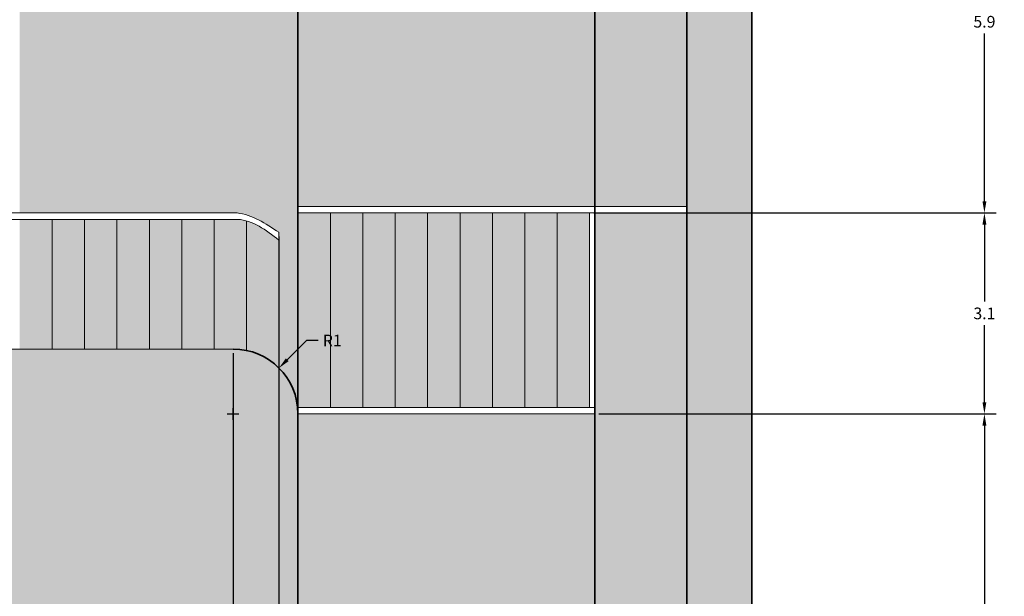
# Model space of a CAD drawing. Units: inches. Extents: x 18 to 59.8, y 2.7 to 81.2.
# Tile 9 of 9: x 44.6 to 59.8, y 45.6 to 54.5. Entities that reach past the tile are written whole.
import ezdxf

# ---------------------------------------------------------------- set-up
doc = ezdxf.new("R2010")
doc.units = ezdxf.units.IN
doc.header["$MEASUREMENT"] = 0
for name, color, linetype, lineweight in [('A-ANNO-DIMS', 2, 'Continuous', 18), ('A-ELEV', 7, 'Continuous', 35), ('A-ELEV-PATT', 8, 'Continuous', 13), ('A-ELEV-RAIL', 7, 'Continuous', 18)]:
    doc.layers.add(name, color=color, linetype=linetype, lineweight=lineweight)
doc.styles.get("Standard").update_dxf_attribs({"font": 'arial.ttf'})
doc.dimstyles.get("Standard").update_dxf_attribs({"dimtxt": 0.18, "dimasz": 0.18, "dimexe": 0.18, "dimexo": 0.0625, "dimgap": 0.09, "dimtad": 0, "dimtih": 1, "dimtoh": 1, "dimdec": 1, "dimzin": 0, "dimdsep": 46, "dimlunit": 3, "dimtxsty": 'Standard', "dimcen": 0.09, "dimadec": 0, "dimazin": 0, "dimtfac": 1, "dimtdec": 1, "dimtofl": 0, "dimtmove": 0, "dimatfit": 3, "dimfxl": 1, "dimtolj": 1, "dimtzin": 0, "dimarcsym": 0})

# ---------------------------------------------------------------- blocks, each defined once
blk = doc.blocks.new('*D17')
at = {"layer": 'A-ANNO-DIMS', "color": 0, "lineweight": -2, "transparency": 16777216}
for p, q in [((53.50256100000002, 48.44074800000003), (59.62997100000005, 48.44074800000003)), ((59.44997100000005, 48.26074800000003), (59.44997100000005, 43.74455863778991)), ((59.44997100000005, 38.86456300000001), (59.44997100000005, 43.38075236221011)), ((53.50256100000002, 38.68456300000001), (59.62997100000006, 38.68456300000001))]:
    blk.add_line(p, q, dxfattribs=at)
at = {"layer": 'A-ANNO-DIMS', "color": 0, "transparency": 16777216}
for points in [[(59.41997100000005, 48.26074800000003), (59.47997100000005, 48.26074800000003), (59.44997100000005, 48.44074800000003)], [(59.41997100000005, 38.86456300000001), (59.47997100000005, 38.86456300000001), (59.44997100000005, 38.68456300000001)]]:
    blk.add_solid(points, dxfattribs=at)
at = {"layer": 'Defpoints', "color": 0, "transparency": 16777216}
for p in [(53.44006100000003, 48.44074800000003), (59.44997100000005, 48.44074800000003), (53.44006100000003, 38.68456300000001)]:
    blk.add_point(p, dxfattribs=at)
at = {"layer": 'A-ANNO-DIMS', "color": 0, "transparency": 16777216, "insert": (59.44997100000005, 43.56265549999998), "char_height": 0.18, "attachment_point": 5}
blk.add_mtext('\\A1;9.756', dxfattribs=at)
blk = doc.blocks.new('*D18')
at = {"layer": 'A-ANNO-DIMS', "color": 0, "lineweight": -2, "transparency": 16777216}
for p, q in [((53.42247100000003, 51.54074800000003), (59.62997100000006, 51.54074800000003)), ((59.44997100000005, 51.36074800000002), (59.44997100000005, 50.17271252933154)), ((59.44997100000005, 48.62074800000002), (59.44997100000005, 49.80878347066851)), ((53.50256100000002, 48.44074800000003), (59.62997100000006, 48.44074800000003))]:
    blk.add_line(p, q, dxfattribs=at)
at = {"layer": 'A-ANNO-DIMS', "color": 0, "transparency": 16777216}
for points in [[(59.41997100000005, 51.36074800000002), (59.47997100000005, 51.36074800000002), (59.44997100000005, 51.54074800000003)], [(59.41997100000005, 48.62074800000002), (59.47997100000005, 48.62074800000002), (59.44997100000005, 48.44074800000003)]]:
    blk.add_solid(points, dxfattribs=at)
at = {"layer": 'Defpoints', "color": 0, "transparency": 16777216}
for p in [(53.35997100000003, 51.54074800000003), (59.44997100000005, 51.54074800000003), (53.44006100000003, 48.44074800000003)]:
    blk.add_point(p, dxfattribs=at)
at = {"layer": 'A-ANNO-DIMS', "color": 0, "transparency": 16777216, "insert": (59.44997100000005, 49.99074799999998), "char_height": 0.18, "attachment_point": 5}
blk.add_mtext('\\A1;3.1', dxfattribs=at)
blk = doc.blocks.new('*D19')
at = {"layer": 'A-ANNO-DIMS', "color": 0, "lineweight": -2, "transparency": 16777216}
for p, q in [((53.50256100000002, 57.44074800000003), (59.62997100000006, 57.44074800000003)), ((59.44997100000005, 57.26074800000002), (59.44997100000005, 54.67265113778992)), ((59.44997100000005, 51.72074800000003), (59.44997100000005, 54.30884486221012)), ((53.42247100000003, 51.54074800000003), (59.62997100000006, 51.54074800000003))]:
    blk.add_line(p, q, dxfattribs=at)
at = {"layer": 'A-ANNO-DIMS', "color": 0, "transparency": 16777216}
for points in [[(59.41997100000005, 57.26074800000002), (59.47997100000005, 57.26074800000002), (59.44997100000005, 57.44074800000003)], [(59.41997100000005, 51.72074800000003), (59.47997100000005, 51.72074800000003), (59.44997100000005, 51.54074800000003)]]:
    blk.add_solid(points, dxfattribs=at)
at = {"layer": 'Defpoints', "color": 0, "transparency": 16777216}
for p in [(53.44006100000003, 57.44074800000003), (59.44997100000005, 57.44074800000003), (53.35997100000003, 51.54074800000003)]:
    blk.add_point(p, dxfattribs=at)
at = {"layer": 'A-ANNO-DIMS', "color": 0, "transparency": 16777216, "insert": (59.44997100000005, 54.49074799999999), "char_height": 0.18, "attachment_point": 5}
blk.add_mtext('\\A1;5.9', dxfattribs=at)
blk = doc.blocks.new('*D51')
at = {"layer": 'A-ANNO-DIMS', "color": 0, "lineweight": -2, "transparency": 16777216}
for p, q in [((34.011642, 44.50324799999999), (34.011642, 81.210748)), ((48.859971, 43.503248), (48.859971, 81.210748)), ((34.191642, 81.03074799999999), (40.98046543587994, 81.03074799999999)), ((48.679971, 81.03074799999999), (41.89114756412005, 81.03074799999999))]:
    blk.add_line(p, q, dxfattribs=at)
at = {"layer": 'A-ANNO-DIMS', "color": 0, "transparency": 16777216}
for points in [[(34.191642, 81.060748), (34.191642, 81.00074799999999), (34.011642, 81.03074799999999)], [(48.679971, 81.060748), (48.679971, 81.00074799999999), (48.859971, 81.03074799999999)]]:
    blk.add_solid(points, dxfattribs=at)
at = {"layer": 'Defpoints', "color": 0, "transparency": 16777216}
for p in [(48.859971, 81.03074799999999), (34.011642, 44.440748), (48.859971, 43.440748)]:
    blk.add_point(p, dxfattribs=at)
at = {"layer": 'A-ANNO-DIMS', "color": 0, "transparency": 16777216, "insert": (41.43580649999999, 81.03074799999999), "char_height": 0.18, "attachment_point": 5}
blk.add_mtext('\\A1;14.848', dxfattribs=at)
blk = doc.blocks.new('*D61')
at = {"layer": 'A-ANNO-DIMS', "color": 0, "lineweight": -2, "transparency": 16777216}
for p, q in [((32.233824, 49.378248), (32.233824, 2.670748000000003)), ((47.859971, 49.378248), (47.859971, 2.670748000000003)), ((32.413824, 2.850747999999999), (39.59180200204638, 2.850747999999999)), ((47.679971, 2.850747999999999), (40.50199299795361, 2.850747999999999))]:
    blk.add_line(p, q, dxfattribs=at)
at = {"layer": 'A-ANNO-DIMS', "color": 0, "transparency": 16777216}
for points in [[(32.413824, 2.880747999999999), (32.413824, 2.820748), (32.233824, 2.850747999999999)], [(47.679971, 2.880747999999999), (47.679971, 2.820748), (47.859971, 2.850747999999999)]]:
    blk.add_solid(points, dxfattribs=at)
at = {"layer": 'Defpoints', "color": 0, "transparency": 16777216}
for p in [(32.233824, 49.440748), (47.859971, 49.440748), (47.859971, 2.850747999999999)]:
    blk.add_point(p, dxfattribs=at)
at = {"layer": 'A-ANNO-DIMS', "color": 0, "transparency": 16777216, "insert": (40.04689749999999, 2.850747999999999), "char_height": 0.18, "attachment_point": 5}
blk.add_mtext('\\A1;15.626', dxfattribs=at)
blk = doc.blocks.new('*D66')
at = {"layer": 'A-ANNO-DIMS', "color": 0, "lineweight": -2, "transparency": 16777216}
for p, q in [((28.803543, 51.378248), (28.803543, 2.670748000000003)), ((48.567078, 51.179103), (48.567078, 2.670748000000003)), ((28.983543, 2.850747999999999), (38.23052195975444, 2.850747999999999)), ((48.387078, 2.850747999999999), (39.14009904024556, 2.850747999999999))]:
    blk.add_line(p, q, dxfattribs=at)
at = {"layer": 'A-ANNO-DIMS', "color": 0, "transparency": 16777216}
for points in [[(28.983543, 2.880747999999999), (28.983543, 2.820748), (28.803543, 2.850747999999999)], [(48.387078, 2.880747999999999), (48.387078, 2.820748), (48.567078, 2.850747999999999)]]:
    blk.add_solid(points, dxfattribs=at)
at = {"layer": 'Defpoints', "color": 0, "transparency": 16777216}
for p in [(28.803543, 51.440748), (48.567078, 51.24160299999999), (48.567078, 2.850747999999999)]:
    blk.add_point(p, dxfattribs=at)
at = {"layer": 'A-ANNO-DIMS', "color": 0, "transparency": 16777216, "insert": (38.6853105, 2.850747999999999), "char_height": 0.18, "attachment_point": 5}
blk.add_mtext('\\A1;19.764', dxfattribs=at)
blk = doc.blocks.new('*D74')
at = {"layer": 'A-ANNO-DIMS', "color": 0, "lineweight": -2, "transparency": 16777216}
for p, q in [((48.99116316341159, 49.57229696346313), (48.69422514902348, 49.27526528903895)), ((49.1711631634116, 49.57229696346313), (48.99116316341159, 49.57229696346313)), ((47.859971, 48.35074800000001), (47.859971, 48.53074800000001)), ((47.769971, 48.44074800000001), (47.949971, 48.44074800000001))]:
    blk.add_line(p, q, dxfattribs=at)
at = {"layer": 'A-ANNO-DIMS', "color": 0, "transparency": 16777216}
blk.add_solid([(48.67300860085032, 49.29647514720953), (48.71544169719663, 49.25405543086837), (48.566966, 49.14796599999999)], dxfattribs=at)
at = {"layer": 'Defpoints', "color": 0, "transparency": 16777216}
for p in [(48.566966, 49.14796599999999), (47.85997100000001, 48.44074800000001)]:
    blk.add_point(p, dxfattribs=at)
at = {"layer": 'A-ANNO-DIMS', "color": 0, "transparency": 16777216, "insert": (49.38891896150163, 49.57229696346313), "char_height": 0.18, "attachment_point": 5}
blk.add_mtext('\\A1;R1', dxfattribs=at)

msp = doc.modelspace()

# ---------------------------------------------------------------- hatches: boundary and pattern name
at = {"layer": 'A-ELEV-PATT'}
h = msp.add_hatch(color=256, dxfattribs=at)
h.set_gradient(color1=(255, 255, 255), color2=(199, 200, 202))
h.paths.add_polyline_path([(38.85997087182833, 75.45212783007513, 0.4125526599533602), (36.85997087192615, 77.44074750583997), (21.85997087182832, 77.44074750583995), (21.85997087182832, 22.44074750583995), (22.85997087182833, 22.44074750583995), (48.85997087182833, 22.44074750583996), (48.85997087182833, 30.92342676155402, 0.4074472928332927), (48.33023903111634, 31.44074750583995), (30.40609029701442, 31.44074750583996, -0.7603989452129261), (34.01164157247843, 44.44074750583996), (47.85997087182832, 44.44074750583995, -0.4142135623730951), (48.85997087182833, 43.44074750583994), (48.85997087182833, 48.44074750583995, 0.4142135623730955), (47.85997087182832, 49.44074750583995), (32.23382408177119, 49.44074750583993, -0.2243141867862321), (27.84111392101349, 52.84266085519661, -0.8480128940945467), (38.85997087182833, 61.44074750583993)])
h.paths.add_polyline_path([(55.85997087182832, 77.44074750583995), (54.85997087182832, 77.44074750583997), (54.85997087182832, 22.24074750583996), (55.85997087182832, 22.24074750583995)])
h.paths.add_polyline_path([(54.85997087182832, 51.54074750583995), (53.44006084017791, 51.54074750583996), (53.44006084017792, 29.64074750583996), (54.85997087182832, 29.64074750583996)])
h.paths.add_polyline_path([(54.85997087182832, 61.44074750583993), (53.44006084017791, 57.44074750583993), (53.44006084017791, 51.64074750583996), (54.85997087182832, 51.64074750583996)])
h.paths.add_polyline_path([(54.85997087182832, 29.44074750583995), (54.47100875861361, 29.44074750583995), (54.47100875861361, 22.24074750583996), (54.85997087182832, 22.24074750583996)])
h.paths.add_polyline_path([(55.57447446325177, 22.24074750583995), (54.85997087182832, 22.24074750583996), (54.57447446325178, 22.24074750583996), (53.93466996146642, 21.792542566958), (54.58769880335594, 21.54947740208223)])
h.paths.add_polyline_path([(54.59913950424823, 21.54521903603421), (53.94430429933965, 21.78895655088426), (53.94430429933965, 18.44074750583995), (54.59913950424823, 18.44074750583995)])
h.paths.add_polyline_path([(53.94430429933965, 21.78895655088427), (53.93466996146642, 21.792542566958), (53.58162006229036, 21.54521903603422), (53.58162006229036, 18.44074750583995), (53.94430429933965, 18.44074750583994)])
h.paths.add_polyline_path([(53.36475139777029, 20.69276091189374), (52.89555240690669, 21.06460517556268), (52.89555240690669, 18.44074750583995), (53.3647513977703, 18.44074750583994)])
h.paths.add_polyline_path([(52.89555240690669, 21.06460517556268), (50.57752474318004, 19.44074750583995), (50.57752474318004, 18.44074750583995), (52.89555240690669, 18.44074750583995)])
h.paths.add_polyline_path([(53.58162006229036, 21.54521903603423), (52.89555240690668, 21.06460517556268), (53.3647513977703, 20.69276091189373), (53.58162006229036, 20.84468482967704)])
h.paths.add_polyline_path([(26.81093959479239, 19.44074750583995), (24.96715419074249, 20.84074750583995), (24.96715419074249, 18.44074750583995), (26.81093959479239, 18.44074750583995)])
h.paths.add_polyline_path([(24.96715419074249, 20.84074750583995), (24.41645576890079, 20.84268308307895), (24.41645576890079, 18.44074750583994), (24.96715419074249, 18.44074750583994)])
h.paths.add_polyline_path([(24.41645576890079, 20.84268308307895), (24.41645576890079, 21.25889692219009), (24.05877847081848, 21.5304839605815), (24.03006070560372, 21.51834150822755), (24.03006070560372, 18.44074750583995), (24.41645576890079, 18.44074750583995)])
h.paths.add_polyline_path([(24.03006070560372, 21.51834150822755), (23.41645576890078, 21.2588969221901), (23.41645576890078, 18.44074750583996), (24.03006070560372, 18.44074750583995)])
h.paths.add_polyline_path([(24.03006070560372, 21.51834150822755), (24.05877847081849, 21.53048396058151), (23.12336878669258, 22.24074750583995), (22.12336878669259, 22.24074750583996), (23.41645576890079, 21.2588969221901)])
h.paths.add_polyline_path([(24.41645576890079, 21.2588969221901), (24.41645576890079, 20.84268308307896), (24.96715419074249, 20.84074750583994)])
h.paths.add_polyline_path([(47.85997087182832, 18.44074750583995), (29.85997087182832, 18.44074750583995), (29.85997087182832, 6.440747505839951), (30.85997087182832, 6.440747505839937), (30.85997087182832, 17.44074750583995), (38.85997087182833, 17.44074750583995), (46.85997087182832, 17.44074750583995), (46.85997087182832, 6.440747505839937), (47.85997087182832, 6.440747505839958)])
h.paths.add_polyline_path([(54.57559250001032, 15.2149800477124), (54.57559250001032, 6.440747505839944), (55.85997087182832, 6.440747505839951), (55.85997087182832, 18.44074750583995), (47.85997087182832, 18.44074750583995), (47.85997087182832, 6.440747505839944), (49.14824210254597, 6.440747505839944), (49.14824210254597, 15.2149800477124, -1)])
h = msp.add_hatch(color=256, dxfattribs=at)
h.paths.add_polyline_path([(27.84111392101356, 52.84266085519647, -0.7443789445921651), (36.85997087182832, 61.44074750583993), (38.85997087182833, 61.44074750583993, 0.8480128940945556)])
h.paths.add_polyline_path([(47.85997087182832, 44.44074750583995), (34.01164157247843, 44.44074750583996, 0.7603989452129407), (30.40609029701462, 31.44074750583983, -0.7376245609052545), (34.01164157247731, 43.44074750583994), (47.85997087182831, 43.44074750583994, -0.4142135623730951), (48.85997087182832, 42.44074750583995), (48.85997087182833, 43.44074750583994, 0.4142135623730951)])
h.paths.add_polyline_path([(54.57559250001032, 15.2149800477124), (54.57559250001032, 6.440747505839951), (55.85997087182832, 6.440747505839951), (55.85997087182832, 18.44074750583995), (47.85997087182832, 18.44074750583995), (47.85997087182832, 6.440747505839944), (49.14824210254597, 6.440747505839944), (49.14824210254597, 15.2149800477124, -1)])
h.paths.add_polyline_path([(47.85997087182832, 18.44074750583995), (29.85997087182832, 18.44074750583995), (29.85997087182832, 6.440747505839958), (30.85997087182832, 6.440747505839951), (30.85997087182832, 17.44074750583995), (38.85997087182833, 17.44074750583995), (46.85997087182832, 17.44074750583995), (46.85997087182832, 6.440747505839944), (47.85997087182832, 6.440747505839951)])
h.paths.add_polyline_path([(55.85997087182832, 77.44074750583995), (54.85997087182832, 77.44074750583997), (54.85997087182833, 22.24074750583995), (55.85997087182832, 22.24074750583995)])
h = msp.add_hatch(dxfattribs=at)
h.set_pattern_fill('ANSI31', color=256, scale=5, angle=45, style=0)
h.set_pattern_definition([(90, (0, 0), (-0.6250000000000001, 0), [])])
h.paths.add_polyline_path([(54.85997087182832, 69.44074750583995), (38.85997087182833, 69.44074750583995), (38.85997087182833, 61.44074750583995), (54.85997087182832, 61.44074750583994)])
h.paths.add_polyline_path([(54.85997087182833, 61.44074750583994), (38.85997087182833, 61.44074750583995), (36.85997087182832, 61.44074750583993, 0.4434140223301819), (27.69861713021859, 58.44074750583995), (48.85997087182833, 58.44074750583995), (48.85997087182833, 57.44074750583994), (53.44006084017792, 57.44074750583995)])
h.paths.add_polyline_path([(37.16613704638868, 59.85769359025997), (37.11866134610267, 59.85769359025997), (37.11866134610267, 59.93991004599954), (37.49943513222304, 59.93991004599954), (37.49943513222304, 59.85769359025997), (37.45195943193702, 59.85769359025997, -3.476462016968403)], flags=16)
h.paths.add_polyline_path([(42.66000754223224, 59.8390978600294), (42.61253184194623, 59.8390978600294), (42.61253184194623, 59.92131431576897), (42.9933056280666, 59.92131431576897), (42.9933056280666, 59.8390978600294), (42.94582992778058, 59.8390978600294, -3.47646201696846)], flags=16)
h.paths.add_polyline_path([(49.64399186138049, 60.00882068949565), (49.59651616109447, 60.00882068949565), (49.59651616109447, 60.09103714523522), (49.97728994721485, 60.09103714523522), (49.97728994721485, 60.00882068949565), (49.92981424692883, 60.00882068949565, -3.476462016968434)], flags=16)
h.paths.add_polyline_path([(44.46707765301489, 57.04074750583994), (32.6670776530149, 57.04074750583994), (32.6670776530149, 56.04074750583993), (44.46707765301489, 56.04074750583993)])
h.paths.add_polyline_path([(47.85997087182831, 43.44074750583994), (46.85997087182832, 43.44074750583994), (34.0116415724774, 43.44074750583994, 0.2012982920418866), (29.34810857035394, 41.44074750583995), (47.85997087182831, 41.44074750583995, 1)])
h.paths.add_polyline_path([(36.60163289663952, 42.55241488062237), (36.55415719635351, 42.55241488062236), (36.55415719635351, 42.63463133636193), (36.93493098247388, 42.63463133636193), (36.93493098247388, 42.55241488062236), (36.88745528218787, 42.55241488062236, -3.476462016968307)], flags=16)
h.paths.add_polyline_path([(42.98647563665846, 42.5780367704526), (42.93899993637245, 42.5780367704526), (42.93899993637245, 42.66025322619216), (43.31977372249282, 42.66025322619216), (43.31977372249282, 42.57803677045259), (43.2722980222068, 42.57803677045259, -3.476462016968351)], flags=16)
h.paths.add_polyline_path([(54.47100875861361, 29.44074750583995), (48.85997087182833, 29.44074750583995), (48.85997087182833, 22.24074750583995), (54.47100875861361, 22.24074750583994)])
h.paths.add_polyline_path([(54.57447446325179, 22.24074750583995), (23.12336878669258, 22.24074750583995), (26.81093959479238, 19.44074750583996), (50.57752474318005, 19.44074750583996)])
h.paths.add_polyline_path([(54.57559250001032, 15.2149800477124, 1), (49.14824210254597, 15.2149800477124), (49.14824210254597, 6.440747505839958), (54.57559250001032, 6.440747505839944)])
h.paths.add_polyline_path([(49.83226884926398, 9.122455521673542), (49.66565363924473, 9.122455521673537), (49.66565363924473, 12.60204276083839), (49.83226884926398, 12.6020427608384)], flags=16)
at = {"layer": 'A-ELEV-PATT', "transparency": 33554620}
h = msp.add_hatch(color=256, dxfattribs=at)
h.set_gradient(color1=(147, 149, 152))
edge = h.paths.add_edge_path()
edge.add_line((32.5670776530149, 55.94074750583994), (32.5670776530149, 57.14074750583994))
edge.add_line((32.5670776530149, 57.14074750583994), (44.5670776530149, 57.14074750583994))
edge.add_line((44.5670776530149, 57.14074750583994), (44.5670776530149, 55.94074750583994))
edge.add_line((44.5670776530149, 55.94074750583994), (44.56707765301487, 51.54074750583998))
edge.add_line((44.56707765301487, 51.54074750583998), (47.92075940082271, 51.54074750583998))
edge.add_spline(control_points=[(47.92075940082271, 51.54074750583998), (48.15238228194087, 51.51452682454292), (48.35972996747788, 51.37806491819363), (48.56707765301488, 51.24160301184435)], knot_values=[0, 0, 0, 0, 0.7121900809507601, 0.7121900809507601, 0.7121900809507601, 0.7121900809507601], degree=3, periodic=0)
edge.add_line((48.56707765301488, 51.24160301184435), (48.56707765301488, 49.14785428702649))
edge.add_arc((47.85997087182832, 48.44074750583995), 1, 5.739170477267294, 44.999999999999375, ccw=False)
edge.add_line((48.85495830893494, 48.54074750583996), (48.85997087182833, 48.54074750583996))
edge.add_line((48.85997087182833, 48.54074750583996), (48.85997087182833, 49.44074750583995))
edge.add_line((48.85997087182833, 49.44074750583995), (48.85997087182833, 58.44074750583995))
edge.add_line((48.85997087182833, 58.44074750583995), (27.6986171302186, 58.44074750583995))
edge.add_arc((33.63815495998532, 55.79107886226907), 6.503756879831279, 155.9580213816849, 220.80747886606)
edge.add_line((28.71539791616241, 51.54074750583994), (32.5670776530149, 51.54074750583994))
edge.add_line((32.5670776530149, 51.54074750583994), (32.5670776530149, 55.94074750583994))
edge = h.paths.add_edge_path()
edge.add_line((32.33023903111487, 40.44074750583996), (35.33023903111486, 40.44074750583996))
edge.add_line((35.33023903111486, 40.44074750583996), (38.33023903111485, 40.44074750583996))
edge.add_line((38.33023903111485, 40.44074750583996), (41.33023903111483, 40.44074750583996))
edge.add_line((41.33023903111483, 40.44074750583996), (44.33023903111482, 40.44074750583996))
edge.add_line((44.33023903111482, 40.44074750583996), (44.33023903111482, 33.83364072465343))
edge.add_line((44.33023903111482, 33.83364072465343), (47.68392077892264, 33.83364072465344))
edge.add_spline(control_points=[(47.68392077892267, 33.83364072465344), (47.91554366004082, 33.80742004335637), (48.12289134557783, 33.67095813700708), (48.33023903111483, 33.5344962306578)], knot_values=[0, 0, 0, 0, 0.7121900809507601, 0.7121900809507601, 0.7121900809507601, 0.7121900809507601], degree=3, periodic=0)
edge.add_line((48.33023903111483, 33.5344962306578), (48.33023903111483, 31.44074750583995))
edge.add_arc((48.3303844405005, 30.91101568508362), 0.5297318407134953, 1.3425044870115812, 90.01572747485528, ccw=False)
edge.add_line((48.85997087182833, 30.92342676155392), (48.85997087182833, 38.68456317332766))
edge.add_line((48.85997087182833, 38.68456317332766), (50.79297551695841, 38.68456317332766))
edge.add_line((50.79297551695841, 38.68456317332766), (50.79297551695841, 41.31595823441438))
edge.add_line((50.79297551695841, 41.31595823441438), (52.92696622669824, 41.31595823441438))
edge.add_line((52.92696622669824, 41.31595823441438), (52.92696622669824, 38.68456317332766))
edge.add_line((52.92696622669824, 38.68456317332766), (53.44006084017791, 38.68456317332766))
edge.add_line((53.44006084017791, 38.68456317332766), (53.44006084017791, 48.44074750583995))
edge.add_line((53.44006084017791, 48.44074750583995), (48.85997087182833, 48.44074750583995))
edge.add_line((48.85997087182833, 48.44074750583995), (48.85997087182832, 42.44074750583995))
edge.add_arc((47.85997087182831, 42.44074750583995), 1, -90, 0, ccw=False)
edge.add_line((47.85997087182831, 41.44074750583995), (29.34810857035394, 41.44074750583995))
edge.add_arc((34.06310194306089, 36.8836189221075), 6.557330511217327, 135.9754091201121, 207.7183105881144)
edge.add_line((28.25825772220566, 33.83364072465339), (32.33023903111487, 33.83364072465341))
edge.add_line((32.33023903111487, 33.83364072465341), (32.33023903111487, 40.44074750583996))
h.paths.add_polyline_path([(53.44006084017791, 57.44074750583995), (48.85997087182833, 57.44074750583994), (48.85997087182833, 51.64074750583996), (53.44006084017791, 51.64074750583996)])
h.paths.add_polyline_path([(29.56707765301488, 51.44074750583992), (28.80354322363853, 51.44074750583992, 0.040450980236505), (29.56707765301488, 50.71907894974708)], flags=17)
h.paths.add_polyline_path([(30.06707765301488, 51.44074750583992), (29.56707765301488, 51.44074750583992), (29.56707765301488, 50.71907894974708, 0.0237787432624053), (30.06707765301488, 50.35543166808938)], flags=17)
h.paths.add_polyline_path([(30.56707765301487, 51.44074750583993), (30.06707765301488, 51.44074750583992), (30.06707765301488, 50.35543166808938, 0.0223728768734236), (30.56707765301488, 50.05807461261393)], flags=17)
h.paths.add_polyline_path([(31.06707765301487, 51.44074750583993), (30.56707765301487, 51.44074750583993), (30.56707765301488, 50.05807461261393, 0.021345047641792), (31.06707765301488, 49.8171007041625)], flags=17)
h.paths.add_polyline_path([(31.56707765301487, 51.44074750583993), (31.06707765301487, 51.44074750583993), (31.06707765301488, 49.8171007041625, 0.0205857748313696), (31.56707765301488, 49.62589497689267)], flags=17)
h.paths.add_polyline_path([(32.06707765301488, 51.44074750583993), (31.56707765301487, 51.44074750583993), (31.56707765301488, 49.62589497689267, 0.0200299041308402), (32.06707765301488, 49.47993240164282)], flags=17)
h.paths.add_polyline_path([(32.5670776530149, 51.44074750583993), (32.06707765301488, 51.44074750583993), (32.06707765301488, 49.47993240164282, 0.0065845078177353), (32.23382408177119, 49.44074750583993), (32.5670776530149, 49.44074750583993)], flags=17)
h.paths.add_polyline_path([(45.06707765301486, 51.44074750583996), (44.56707765301487, 51.44074750583996), (44.56707765301487, 49.44074750583995), (45.06707765301488, 49.44074750583995)], flags=17)
h.paths.add_polyline_path([(45.56707765301488, 51.44074750583996), (45.06707765301486, 51.44074750583996), (45.06707765301488, 49.44074750583995), (45.56707765301488, 49.44074750583995)], flags=17)
h.paths.add_polyline_path([(46.06707765301488, 51.44074750583996), (45.56707765301488, 51.44074750583996), (45.56707765301488, 49.44074750583995), (46.06707765301488, 49.44074750583995)], flags=17)
h.paths.add_polyline_path([(46.56707765301487, 51.44074750583996), (46.06707765301488, 51.44074750583996), (46.06707765301488, 49.44074750583995), (46.56707765301487, 49.44074750583995)], flags=17)
h.paths.add_polyline_path([(47.06707765301487, 51.44074750583996), (46.56707765301487, 51.44074750583996), (46.56707765301487, 49.44074750583995), (47.06707765301487, 49.44074750583995)], flags=17)
h.paths.add_polyline_path([(47.56707765301487, 51.44074750583996), (47.06707765301487, 51.44074750583996), (47.06707765301487, 49.44074750583995), (47.56707765301488, 49.44074750583995)], flags=17)
edge = h.paths.add_edge_path(flags=17)
edge.add_spline(control_points=[(48.06707765301273, 51.41840713962396), (48.02172392661717, 51.43105064440995), (47.97524027779975, 51.4389035969284), (47.92733930740307, 51.44074750583996)], knot_values=[0.5701039528936005, 0.5701039528936005, 0.5701039528936005, 0.5701039528936005, 0.7151116034373463, 0.7151116034373463, 0.7151116034373463, 0.7151116034373644], degree=3, periodic=0)
edge.add_line((47.92733930740307, 51.44074750583996), (47.56707765301487, 51.44074750583996))
edge.add_line((47.56707765301487, 51.44074750583996), (47.56707765301488, 49.44074750583995))
edge.add_line((47.56707765301488, 49.44074750583995), (47.85997087182832, 49.44074750583995))
edge.add_arc((47.85997087182832, 48.44074750583995), 1, 78.04714410929728, 90, ccw=False)
edge.add_line((48.06707765301489, 49.41906584931846), (48.06707765301488, 51.41840713962341))
edge = h.paths.add_edge_path(flags=17)
edge.add_spline(control_points=[(48.56707765301488, 51.12118615879595), (48.40623273758901, 51.24494240176197), (48.24538782216315, 51.36869864472799), (48.06707765301273, 51.41840713962396)], knot_values=[0, 0, 0, 0, 0.5701039528936005, 0.5701039528936005, 0.5701039528936005, 0.5701039528936005], degree=3, periodic=0)
edge.add_line((48.06707765301488, 51.41840713962327), (48.06707765301489, 49.41906584931846))
edge.add_arc((47.85997087182832, 48.44074750583995), 1, 44.999999999999375, 78.04714410929728, ccw=False)
edge.add_line((48.56707765301488, 49.14785428702649), (48.56707765301488, 51.12118615879595))
h.paths.add_polyline_path([(49.35997087182833, 51.54074750583996), (48.85997087182833, 51.54074750583996), (48.85997087182833, 49.44074750583995), (48.85997087182833, 48.54074750583996), (49.35997087182833, 48.54074750583996)])
h.paths.add_polyline_path([(49.85997087182834, 51.54074750583996), (49.35997087182833, 51.54074750583996), (49.35997087182833, 48.54074750583996), (49.85997087182833, 48.54074750583996)])
h.paths.add_polyline_path([(50.35997087182834, 51.54074750583996), (49.85997087182834, 51.54074750583996), (49.85997087182833, 48.54074750583996), (50.35997087182833, 48.54074750583996)])
h.paths.add_polyline_path([(50.85997087182834, 51.54074750583996), (50.35997087182834, 51.54074750583996), (50.35997087182832, 48.54074750583996), (50.85997087182833, 48.54074750583996)])
h.paths.add_polyline_path([(51.35997087182833, 51.54074750583996), (50.85997087182834, 51.54074750583996), (50.85997087182833, 48.54074750583996), (51.35997087182833, 48.54074750583996)])
h.paths.add_polyline_path([(51.85997087182833, 51.54074750583996), (51.35997087182833, 51.54074750583996), (51.35997087182833, 48.54074750583995), (51.85997087182832, 48.54074750583995)])
h.paths.add_polyline_path([(52.35997087182834, 51.54074750583995), (51.85997087182833, 51.54074750583996), (51.85997087182832, 48.54074750583995), (52.35997087182834, 48.54074750583995)])
h.paths.add_polyline_path([(52.85997087182835, 51.54074750583995), (52.35997087182834, 51.54074750583995), (52.35997087182834, 48.54074750583995), (52.85997087182833, 48.54074750583995)])
h.paths.add_polyline_path([(53.35997087182834, 51.54074750583995), (52.85997087182835, 51.54074750583995), (52.85997087182833, 48.54074750583995), (53.35997087182834, 48.54074750583995)])
h.paths.add_polyline_path([(53.44006084017792, 38.68456317332766), (48.85997087182833, 38.68456317332766), (48.85997087182833, 30.92342676155392), (48.85997087182833, 29.64074750583995), (53.44006084017792, 29.64074750583994)])
h.paths.add_polyline_path([(28.83023903111483, 33.73364072465339), (28.31190895474052, 33.73364072465339, 0.0364451520675395), (28.83023903111484, 32.93194469741221)], flags=17)
h.paths.add_polyline_path([(29.33023903111483, 33.73364072465339), (28.83023903111483, 33.73364072465339), (28.83023903111484, 32.9319446974122, 0.0294200839082379), (29.33023903111484, 32.34505173740402)], flags=17)
h.paths.add_polyline_path([(29.83023903111483, 33.73364072465339), (29.33023903111483, 33.73364072465339), (29.33023903111484, 32.34505173740402, 0.0261691093073466), (29.83023903111483, 31.87548004603654)], flags=17)
h.paths.add_polyline_path([(30.33023903111483, 33.73364072465339), (29.83023903111483, 33.73364072465339), (29.83023903111483, 31.87548004603654, 0.0240262665661449), (30.33023903111483, 31.49248565404972)], flags=17)
h.paths.add_polyline_path([(30.83023903111483, 33.73364072465339), (30.33023903111483, 33.73364072465339), (30.33023903111483, 31.49248565404973, 0.0035005678246481), (30.40609029701443, 31.44074750583996), (30.83023903111484, 31.44074750583996)], flags=17)
h.paths.add_polyline_path([(31.33023903111483, 33.73364072465339), (30.83023903111483, 33.73364072465339), (30.83023903111484, 31.44074750583996), (31.33023903111483, 31.44074750583996)], flags=17)
h.paths.add_polyline_path([(31.83023903111483, 33.73364072465339), (31.33023903111483, 33.73364072465339), (31.33023903111483, 31.44074750583996), (31.83023903111483, 31.44074750583996)], flags=17)
h.paths.add_polyline_path([(32.33023903111487, 33.7336407246534), (31.83023903111483, 33.7336407246534), (31.83023903111483, 31.44074750583996), (32.33023903111487, 31.44074750583996)], flags=17)
h.paths.add_polyline_path([(44.83023903111482, 33.73364072465341), (44.33023903111482, 33.73364072465341), (44.33023903111482, 31.44074750583995), (44.83023903111483, 31.44074750583995)], flags=17)
h.paths.add_polyline_path([(45.33023903111483, 33.73364072465341), (44.83023903111482, 33.73364072465341), (44.83023903111483, 31.44074750583996), (45.33023903111483, 31.44074750583995)], flags=17)
h.paths.add_polyline_path([(45.83023903111483, 33.73364072465341), (45.33023903111483, 33.73364072465341), (45.33023903111483, 31.44074750583996), (45.83023903111483, 31.44074750583995)], flags=17)
h.paths.add_polyline_path([(46.33023903111483, 33.73364072465342), (45.83023903111483, 33.73364072465342), (45.83023903111483, 31.44074750583995), (46.33023903111482, 31.44074750583996)], flags=17)
h.paths.add_polyline_path([(46.83023903111482, 33.73364072465342), (46.33023903111483, 33.73364072465342), (46.33023903111482, 31.44074750583996), (46.83023903111482, 31.44074750583995)], flags=17)
h.paths.add_polyline_path([(47.33023903111482, 33.73364072465342), (46.83023903111482, 33.73364072465341), (46.83023903111482, 31.44074750583996), (47.33023903111484, 31.44074750583996)], flags=17)
edge = h.paths.add_edge_path(flags=16)
edge.add_spline(control_points=[(47.83023903111267, 33.71130035843739), (47.78488530471712, 33.7239438632234), (47.7384016558997, 33.73179681574185), (47.690500685503, 33.73364072465343)], knot_values=[0.5701039528936152, 0.5701039528936152, 0.5701039528936152, 0.5701039528936152, 0.7151116034373552, 0.7151116034373552, 0.7151116034373552, 0.7151116034373644], degree=3, periodic=0)
edge.add_line((47.69050068550314, 33.73364072465342), (47.33023903111482, 33.73364072465342))
edge.add_line((47.33023903111482, 33.73364072465342), (47.33023903111484, 31.44074750583995))
edge.add_line((47.33023903111484, 31.44074750583995), (47.83023903111484, 31.44074750583995))
edge.add_line((47.83023903111484, 31.44074750583995), (47.83023903111483, 33.71130035843684))
h.paths.add_polyline_path([(48.85997087182833, 38.68456317332766), (50.79297551695841, 38.68456317332766), (50.79297551695841, 41.31595823441438), (52.92696622669824, 41.31595823441438), (52.92696622669824, 38.68456317332766), (53.44006084017791, 38.68456317332766), (53.44006084017791, 48.44074750583995), (48.85997087182833, 48.44074750583995), (48.85997087182832, 42.44074750583995, -0.414213562373094), (47.85997087182831, 41.44074750583995), (29.34810857035394, 41.44074750583995, 0.3236799116418651), (28.25825772220566, 33.83364072465339), (32.33023903111487, 33.83364072465341), (32.33023903111487, 40.44074750583996), (35.33023903111486, 40.44074750583996), (38.33023903111485, 40.44074750583996), (41.33023903111483, 40.44074750583996), (44.33023903111482, 40.44074750583996), (44.33023903111482, 33.83364072465343), (28.25825772220566, 33.83364072465339, 0.0043266617348909), (28.31190895474052, 33.73364072465339), (28.83023903111483, 33.73364072465339), (29.33023903111483, 33.73364072465339), (29.83023903111483, 33.73364072465339), (30.33023903111483, 33.73364072465339), (30.83023903111483, 33.73364072465339), (31.33023903111483, 33.73364072465339), (31.83023903111483, 33.73364072465339), (32.33023903111487, 33.7336407246534), (47.33023903111482, 33.73364072465342), (47.33023903111484, 31.44074750583995), (47.83023903111484, 31.44074750583995), (48.33023903111591, 31.44074750583995, -0.4074472928335827), (48.85997087182833, 30.92342676155392)])
edge = h.paths.add_edge_path(flags=0)
edge.add_spline(control_points=[(47.83023903111267, 33.71130035843739), (47.78488530471713, 33.7239438632234), (47.73840165589972, 33.73179681574185), (47.69050068550303, 33.73364072465341)], knot_values=[0.5701039528936152, 0.5701039528936152, 0.5701039528936152, 0.5701039528936152, 0.7151116034373257, 0.7151116034373257, 0.7151116034373257, 0.7151116034373644], degree=3, periodic=0)
edge.add_line((47.69050068550293, 33.73364072465342), (47.33023903111482, 33.73364072465342))
edge.add_line((47.33023903111482, 33.73364072465342), (47.33023903111484, 31.44074750583995))
edge.add_line((47.33023903111484, 31.44074750583995), (47.83023903111484, 31.44074750583995))
edge.add_line((47.83023903111484, 31.44074750583995), (47.83023903111483, 33.71130035843687))
h = msp.add_hatch(color=256, dxfattribs=at)
h.set_gradient(color1=(147, 149, 152))
edge = h.paths.add_edge_path()
edge.add_line((44.33023903111482, 33.83364072465343), (47.68392077892268, 33.83364072465344))
edge.add_spline(control_points=[(47.68392077892267, 33.83364072465344), (47.91554366004082, 33.80742004335637), (48.12289134557783, 33.67095813700708), (48.33023903111483, 33.5344962306578)], knot_values=[0, 0, 0, 0, 0.7121900809507601, 0.7121900809507601, 0.7121900809507601, 0.7121900809507601], degree=3, periodic=0)
edge.add_line((48.33023903111483, 33.5344962306578), (48.33023903111483, 31.44074750583995))
edge.add_arc((48.3303844405005, 30.91101568508362), 0.5297318407134953, 1.3425044870177203, 90.01572747485528, ccw=False)
edge.add_line((48.85997087182833, 30.92342676155398), (48.85997087182833, 38.68456317332766))
edge.add_line((48.85997087182833, 38.68456317332766), (50.79297551695841, 38.68456317332766))
edge.add_line((50.79297551695841, 38.68456317332766), (50.79297551695841, 41.31595823441438))
edge.add_line((50.79297551695841, 41.31595823441438), (52.92696622669824, 41.31595823441438))
edge.add_line((52.92696622669824, 41.31595823441438), (52.92696622669824, 38.68456317332766))
edge.add_line((52.92696622669824, 38.68456317332766), (53.44006084017791, 38.68456317332766))
edge.add_line((53.44006084017791, 38.68456317332766), (53.44006084017791, 48.44074750583995))
edge.add_line((53.44006084017791, 48.44074750583995), (48.85997087182833, 48.44074750583995))
edge.add_line((48.85997087182833, 48.44074750583995), (48.85997087182832, 42.44074750583995))
edge.add_arc((47.85997087182831, 42.44074750583995), 1, -90, 0, ccw=False)
edge.add_line((47.85997087182831, 41.44074750583995), (29.34810857035394, 41.44074750583995))
edge.add_arc((34.06310194306089, 36.8836189221075), 6.557330511217328, 135.9754091201121, 207.7183105881144)
edge.add_line((28.25825772220566, 33.83364072465339), (32.33023903111487, 33.8336407246534))
edge.add_line((32.33023903111487, 33.8336407246534), (32.33023903111487, 40.44074750583996))
edge.add_line((32.33023903111487, 40.44074750583996), (35.33023903111486, 40.44074750583996))
edge.add_line((35.33023903111486, 40.44074750583996), (38.33023903111485, 40.44074750583996))
edge.add_line((38.33023903111485, 40.44074750583996), (41.33023903111483, 40.44074750583996))
edge.add_line((41.33023903111483, 40.44074750583996), (44.33023903111482, 40.44074750583996))
edge.add_line((44.33023903111482, 40.44074750583996), (44.33023903111482, 33.83364072465343))

# ---------------------------------------------------------------- linework, layer by layer
at = {"layer": 'A-ELEV'}
for p, q in [((54.85997087182833, 22.24074750583995), (54.85997087182832, 77.44074750583995)), ((55.85997087182832, 77.44074750583994), (55.85997087182832, 22.24074750583995)), ((48.85997087182833, 42.44074750583995), (48.85997087182833, 58.44074750583994)), ((53.44006084017791, 57.44074750583996), (53.44006084017792, 29.64074750583995))]:
    msp.add_line(p, q, dxfattribs=at)
msp.add_arc((47.85997087182832, 48.44074750583995), 1, 0, 89.99999999999959, dxfattribs=at)
at = {"layer": 'A-ELEV-RAIL'}
for p, q in [((47.9207594008227, 51.54074750583998), (28.71539791616241, 51.54074750583994)), ((54.85997087182834, 51.64074750583996), (48.85997087182834, 51.64074750583996)), ((54.85997087182834, 51.54074750583995), (48.85997087182834, 51.54074750583996)), ((49.35997087182833, 51.54074750583995), (49.35997087182833, 48.54074750583995)), ((49.85997087182834, 51.54074750583995), (49.85997087182833, 48.54074750583995)), ((50.35997087182834, 51.54074750583995), (50.35997087182833, 48.54074750583995)), ((50.85997087182834, 51.54074750583995), (50.85997087182833, 48.54074750583995)), ((51.35997087182833, 51.54074750583995), (51.35997087182833, 48.54074750583995)), ((51.85997087182833, 51.54074750583995), (51.85997087182833, 48.54074750583995)), ((52.35997087182834, 51.54074750583994), (52.35997087182833, 48.54074750583994)), ((52.85997087182834, 51.54074750583994), (52.85997087182833, 48.54074750583994)), ((53.35997087182834, 51.54074750583994), (53.35997087182833, 48.54074750583994)), ((54.85997087182834, 51.54074750583994), (54.85997087182833, 48.54074750583994)), ((47.92733930740303, 51.44074750583996), (28.80354322363853, 51.44074750583992)), ((45.06707765301488, 49.44074750583994), (45.06707765301487, 51.44074750583995)), ((45.56707765301488, 49.44074750583995), (45.56707765301488, 51.44074750583995)), ((46.06707765301488, 49.44074750583995), (46.06707765301488, 51.44074750583996)), ((46.56707765301487, 49.44074750583995), (46.56707765301487, 51.44074750583996)), ((47.06707765301487, 49.44074750583995), (47.06707765301487, 51.44074750583996)), ((47.56707765301488, 49.44074750583995), (47.56707765301487, 51.44074750583996)), ((48.06707765301489, 49.41906584931846), (48.06707765301488, 51.41840713963304)), ((48.56707765301488, 49.1478542870265), (48.56707765301488, 51.24160301184435)), ((47.85997087182832, 49.44074750583995), (32.23382408177118, 49.44074750583993)), ((48.85997087182833, 49.44074750583995), (48.85997087182833, 48.44074750583995)), ((53.44006084017792, 48.54074750583995), (48.85997087182833, 48.54074750583996)), ((53.44006084017792, 48.44074750583995), (48.85997087182833, 48.44074750583995))]:
    msp.add_line(p, q, dxfattribs=at)
msp.add_open_spline([(48.56707765301488, 51.24160301184435), (48.35972996747788, 51.37806491819363), (48.15238228194087, 51.51452682454292), (47.92075940082271, 51.54074750583998)], degree=3, dxfattribs=at)
msp.add_open_spline([(48.56707765301488, 51.12118615879595), (48.36532135086834, 51.27642017338861), (48.14473421419293, 51.44614288553839), (47.88294298389387, 51.44117186622448), (47.86059468465408, 51.44074750583996)], degree=3, knots=[0, 0, 0, 0, 0.7151116034373644, 0.7818562261863207, 0.7818562261863207, 0.7818562261863207, 0.7818562261863207], dxfattribs=at)

# ---------------------------------------------------------------- dimensions: what is measured, and where the dimension line sits
at = {"layer": 'A-ANNO-DIMS'}
for base, p1, p2, picture, middle in [((48.859971, 81.03074799999999), (34.011642, 44.440748), (48.859971, 43.440748), '*D51', (41.43580649999999, 81.03074799999999)), ((48.567078, 2.850747999999999), (28.803543, 51.440748), (48.567078, 51.24160299999999), '*D66', (38.6853105, 2.850747999999999)), ((47.859971, 2.850747999999999), (32.233824, 49.440748), (47.859971, 49.440748), '*D61', (40.04689749999999, 2.850747999999999))]:
    dim = msp.add_linear_dim(base=base, p1=p1, p2=p2, dimstyle='Standard', override={"dimdec": 3, "dimlfac": 1, "dimrnd": 0, "dimzin": 0, "dimdsep": 46, "dimlunit": 2}, dxfattribs=at)
    dim.commit()
    dim.dimension.update_dxf_attribs({"geometry": picture, "text_midpoint": middle})
for base, p1, p2, override, picture, middle in [((59.44997100000005, 57.44074800000003), (53.359971, 51.540748), (53.440061, 57.44074799999999), {"dimdec": 1, "dimlfac": 1, "dimrnd": 0, "dimzin": 0, "dimdsep": 46, "dimlunit": 2}, '*D19', (59.44997100000005, 54.49074799999999)), ((59.44997100000005, 51.54074800000003), (53.440061, 48.440748), (53.359971, 51.540748), {"dimdec": 1, "dimlfac": 1, "dimrnd": 0, "dimzin": 0, "dimdsep": 46, "dimlunit": 2}, '*D18', (59.44997100000005, 49.99074799999998)), ((59.44997100000005, 48.44074800000003), (53.440061, 38.684563), (53.440061, 48.440748), {"dimdec": 3, "dimlfac": 1, "dimrnd": 0, "dimzin": 0, "dimdsep": 46, "dimlunit": 2}, '*D17', (59.44997100000005, 43.56265549999998))]:
    dim = msp.add_linear_dim(base=base, p1=p1, p2=p2, angle=90, dimstyle='Standard', override=override, dxfattribs=at)
    dim.commit()
    dim.dimension.update_dxf_attribs({"geometry": picture, "text_midpoint": middle})
dim = msp.add_radius_dim(center=(47.85997100000001, 48.44074800000001), mpoint=(48.566966, 49.14796599999999), dimstyle='Standard', override={"dimdec": 0, "dimlfac": 1, "dimrnd": 0, "dimzin": 0, "dimdsep": 46, "dimlunit": 2}, dxfattribs=at)
dim.commit()
dim.dimension.update_dxf_attribs({"geometry": '*D74', "text_midpoint": (49.38891896150163, 49.57229696346313), "dimtype": 164})

doc.saveas('drawing.dxf')
